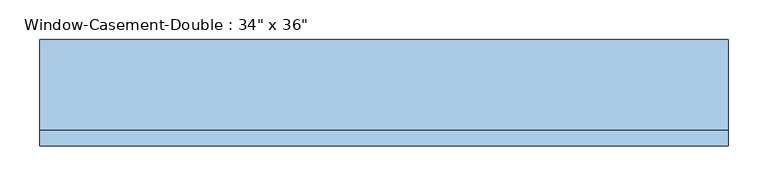
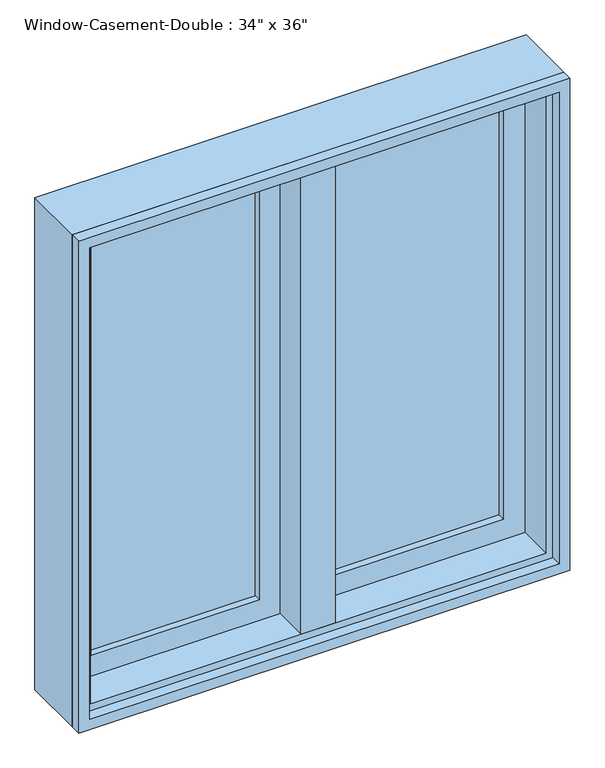
"""IFC4 building model written with IfcOpenShell, lengths in millimetres: window geometry."""

from ifc_helpers import new_model, si_unit, frame, origin, place, context, project, spatial, polyline, outline, extrude, faceted_brep, source, transform, mapped, element, save


def window_a598f463(model_context):
    return source(origin(), model_context, "Body", "SolidModel", [
        faceted_brep([(9.525, 76.2, 1816.1), (-9.525, 76.2, 1816.1), (-9.525, 25.4, 1816.1), (9.525, 25.4, 1816.1), (9.525, 76.2, 927.1), (9.525, 25.4, 927.1), (-9.525, 25.4, 927.1), (-9.525, 76.2, 927.1), (-9.525, 25.4, 946.15), (-9.525, 25.4, 1797.05), (-30.1625, 25.4, 946.15), (-30.1625, 25.4, 1797.05), (-30.1625, -38.1, 946.15), (-30.1625, -38.1, 1797.05), (30.1625, -38.1, 946.15), (30.1625, -38.1, 1797.05), (30.1625, 25.4, 946.15), (30.1625, 25.4, 1797.05), (9.525, 25.4, 946.15), (9.525, 25.4, 1797.05)], [[[0, 1, 2, 3]], [[4, 5, 6, 7]], [[1, 0, 4, 7]], [[2, 1, 7, 6, 8, 9]], [[9, 8, 10, 11]], [[11, 10, 12, 13]], [[13, 12, 14, 15]], [[15, 14, 16, 17]], [[17, 16, 18, 19]], [[0, 3, 19, 18, 5, 4]], [[18, 8, 6, 5]], [[9, 19, 3, 2]], [[8, 18, 16, 14, 12, 10]], [[19, 9, 11, 13, 15, 17]]]),
        extrude(outline(polyline([(-66.675, 57.15), (-66.675, 50.8), (-361.95, 50.8), (-361.95, 57.15), (-66.675, 57.15)])), frame((0.0, 0.0, 984.25), z_axis=(0.0, 0.0, 1.0), x_axis=(1.0, 0.0, 0.0)), (0.0, 0.0, 1.0), 774.7),
        extrude(outline(polyline([(-361.95, 38.1), (-361.95, 44.45), (-66.675, 44.45), (-66.675, 38.1), (-361.95, 38.1)])), frame((0.0, 0.0, 984.25), z_axis=(0.0, 0.0, 1.0), x_axis=(1.0, 0.0, 0.0)), (0.0, 0.0, 1.0), 774.7),
        extrude(outline(polyline([(361.95, 57.15), (361.95, 50.8), (66.675, 50.8), (66.675, 57.15), (361.95, 57.15)])), frame((0.0, 0.0, 984.25), z_axis=(0.0, 0.0, 1.0), x_axis=(1.0, 0.0, 0.0)), (0.0, 0.0, 1.0), 774.7),
        extrude(outline(polyline([(66.675, 38.1), (66.675, 44.45), (361.95, 44.45), (361.95, 38.1), (66.675, 38.1)])), frame((0.0, 0.0, 984.25), z_axis=(0.0, 0.0, 1.0), x_axis=(1.0, 0.0, 0.0)), (0.0, 0.0, 1.0), 774.7),
        extrude(outline(polyline([(1816.1, -419.1), (927.1, -419.1), (927.1, -9.525), (1816.1, -9.525), (1816.1, -419.1)]), holes=[polyline([(1758.95, -66.675), (984.25, -66.675), (984.25, -361.95), (1758.95, -361.95), (1758.95, -66.675)])]), frame((0.0, 25.4, 0.0), z_axis=(0.0, 1.0, 0.0), x_axis=(0.0, 0.0, 1.0)), (0.0, 0.0, 1.0), 44.45),
        extrude(outline(polyline([(927.1, 419.1), (1816.1, 419.1), (1816.1, 9.525), (927.1, 9.525), (927.1, 419.1)]), holes=[polyline([(984.25, 66.675), (1758.95, 66.675), (1758.95, 361.95), (984.25, 361.95), (984.25, 66.675)])]), frame((0.0, 25.4, 0.0), z_axis=(0.0, 1.0, 0.0), x_axis=(0.0, 0.0, 1.0)), (0.0, 0.0, 1.0), 44.45),
        extrude(outline(polyline([(1828.8, -431.8), (914.4, -431.8), (914.4, 431.8), (1828.8, 431.8), (1828.8, -431.8)]), holes=[polyline([(1809.75, 412.75), (933.45, 412.75), (933.45, -412.75), (1809.75, -412.75), (1809.75, 412.75)])]), frame((0.0, -57.15, 0.0), z_axis=(0.0, 1.0, 0.0), x_axis=(0.0, 0.0, 1.0)), (0.0, 0.0, 1.0), 19.05),
        faceted_brep([(400.05, 25.4, 1797.05), (400.05, -38.1, 1797.05), (-400.05, -38.1, 1797.05), (-400.05, 25.4, 1797.05), (419.1, 76.2, 1816.1), (419.1, 25.4, 1816.1), (-419.1, 25.4, 1816.1), (-419.1, 76.2, 1816.1), (431.8, -38.1, 1828.8), (431.8, 76.2, 1828.8), (-431.8, 76.2, 1828.8), (-431.8, -38.1, 1828.8), (-400.05, -38.1, 946.15), (-400.05, 25.4, 946.15), (-419.1, 25.4, 927.1), (-419.1, 76.2, 927.1), (-431.8, 76.2, 914.4), (-431.8, -38.1, 914.4), (400.05, -38.1, 946.15), (400.05, 25.4, 946.15), (419.1, 25.4, 927.1), (419.1, 76.2, 927.1), (431.8, 76.2, 914.4), (431.8, -38.1, 914.4)], [[[0, 1, 2, 3]], [[4, 5, 6, 7]], [[8, 9, 10, 11]], [[3, 2, 12, 13]], [[7, 6, 14, 15]], [[11, 10, 16, 17]], [[13, 12, 18, 19]], [[15, 14, 20, 21]], [[17, 16, 22, 23]], [[11, 17, 23, 8], [1, 18, 12, 2]], [[19, 18, 1, 0]], [[5, 20, 14, 6], [3, 13, 19, 0]], [[21, 20, 5, 4]], [[23, 22, 9, 8]], [[9, 22, 16, 10], [7, 15, 21, 4]]]),
    ])


if __name__ == "__main__":
    model = new_model("IFC4")
    model_context = context("Model", 3, world=origin())
    ifc_project = project(units=[si_unit("LENGTHUNIT", "METRE", prefix="MILLI")], contexts=[model_context])
    site = spatial("IfcSite", under=ifc_project)
    building = spatial("IfcBuilding", under=site)
    placement = place(None, origin())
    window_shape = window_a598f463(model_context)
    element("IfcWindow", 1, ObjectType="Window-Casement-Double : 34\" x 36\"", at=placement, inside=building, context=model_context, shape_type="MappedRepresentation", body=[
        mapped(window_shape, transform((0.0, 0.0, 0.0), x_axis=(1.0, 0.0, 0.0), y_axis=(0.0, 1.0, 0.0), z_axis=(0.0, 0.0, 1.0))),
    ])
    save(model, "model.ifc")

# Revit data of these elements
# Type "Window-Casement-Double : 34\" x 36\""
#   Type Mark = "14"
#   Fire Rating = "0.5h"
#   Assembly Code = "B2020100"
#   Analytic Construction = "Double glazing - domestic"
#   Frame Extension [instance default] = 0' - 0 1/4"
#   Window Inset [instance default] = 0' - 0"
#   Wall Thickness [instance default] = 0' - 6"
#   Interior Wall Closure [instance default] = 0' - 2 1/4"
#   Half Width = 1' - 5"
#   Visual Light Transmittance = 0.81
#   Thermal Resistance (R) = 1.8146 (h·ft²·°F)/BTU
#   Solar Heat Gain Coefficient = 0.76
#   Rough Width = 2' - 10 1/2"
#   Rough Height = 3' - 0 1/2"
#   Height = 3' - 0"
#   Heat Transfer Coefficient (U) = 0.5511 BTU/(h·ft²·°F)
#   Exterior Wall Closure [instance default] = 0' - 1 1/4"
#   Extension Jamb [instance default] = 0' - 2 1/4"
#   Default Sill Height = 3' - 0"
#   Width = 2' - 10"
#   Define Thermal Properties by = 0
#   Muntin Visibility = yes
#   Interior Trim Visibility [instance default] = yes
#   Exterior Trim Visibility [instance default] = yes
#   Extension Jamb Visibility [instance default] = yes
#   Interior Trim Material = Wood - Stained
#   Muntin Pattern = Muntin Pattern_2x2 : Muntin Pattern_2x2
#   Interior Trim = Trim-Window-Interior-Flat : Picture Frame
#   Interior Frame Material = Wood - Stained
#   Glass Panel Material = Glass
#   Exterior Trim Material = Clad - White
#   Exterior Trim = Trim-Window-Exterior-Flat : with Sill
#   Exterior Frame Material = Clad - White
#   Wall Closure = (empty or 0)
# Element 1 (IfcWindow, "Window-Casement-Double : 34\" x 36\"")
#   Wall Thickness = 0' - 4 1/2"
#   Extension Jamb = 0' - 0 3/4"
#   Materials on its faces: "Wood - Stained", "Glass", "Clad - White"
# Materials
#   "Wood - Stained": class "Wood", colour RGB 224 178 126, transparency 0, Cost = 0
#   "Glass": class "Glass", colour RGB 0 128 192, transparency 0.75, Description = "Soda Lime Glass", Cost = 0
#   "Clad - White": class "Wood", colour RGB 242 242 238, transparency 0, Cost = 0
